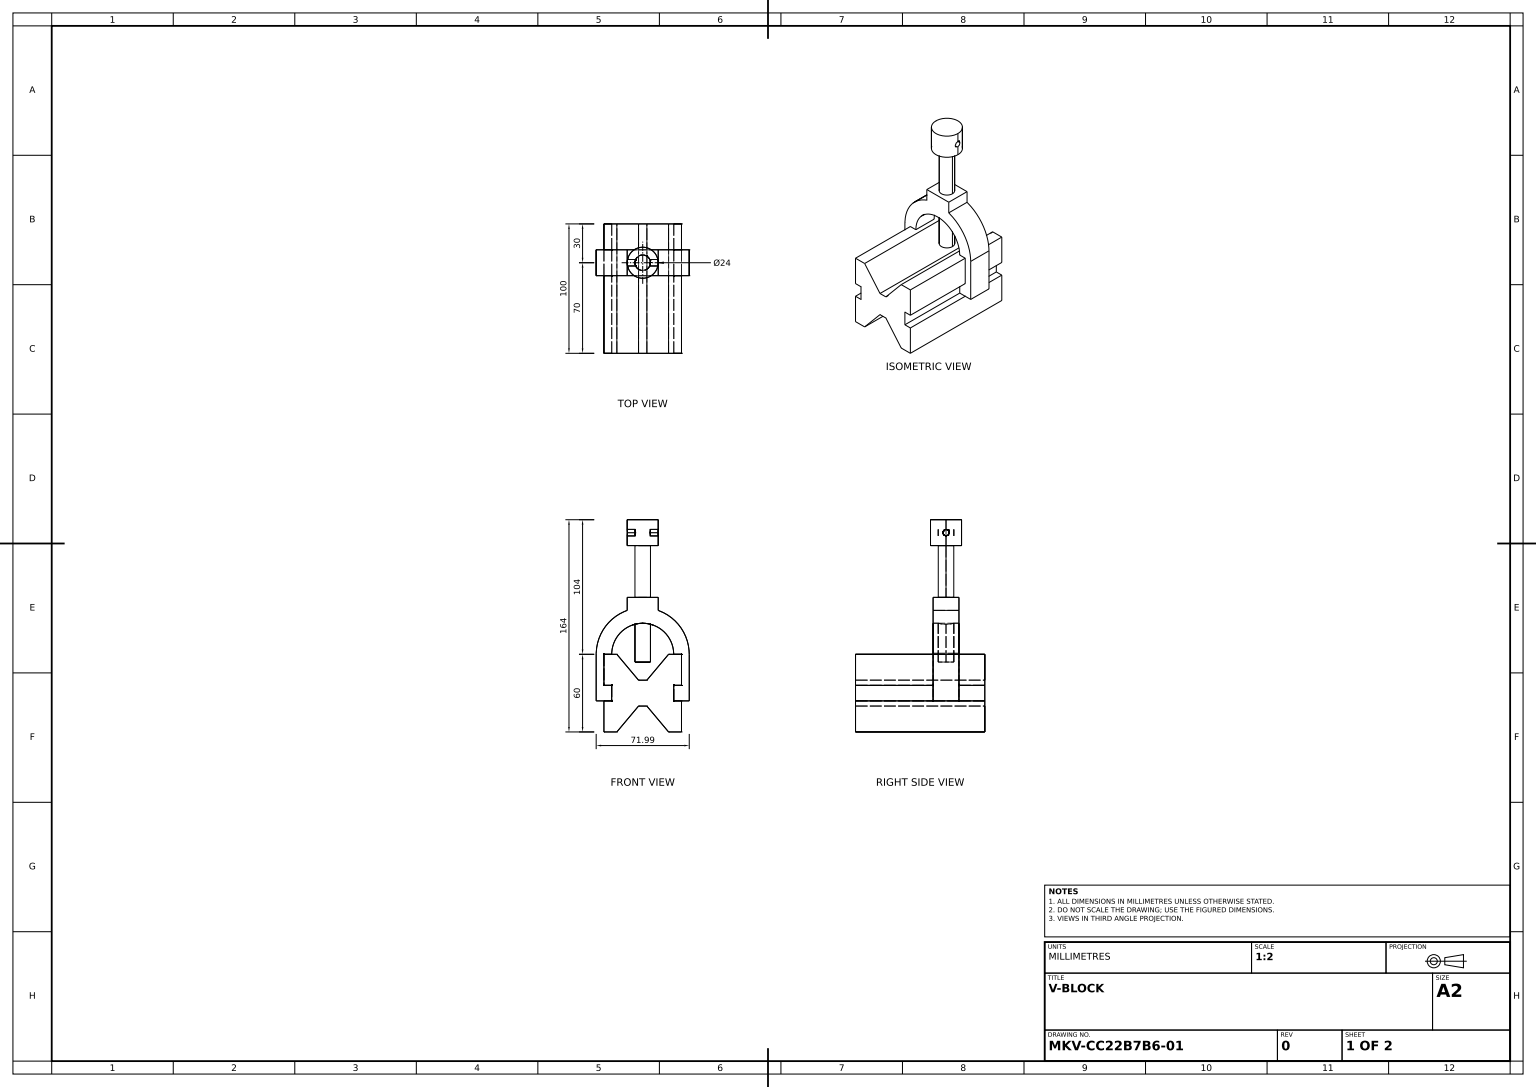
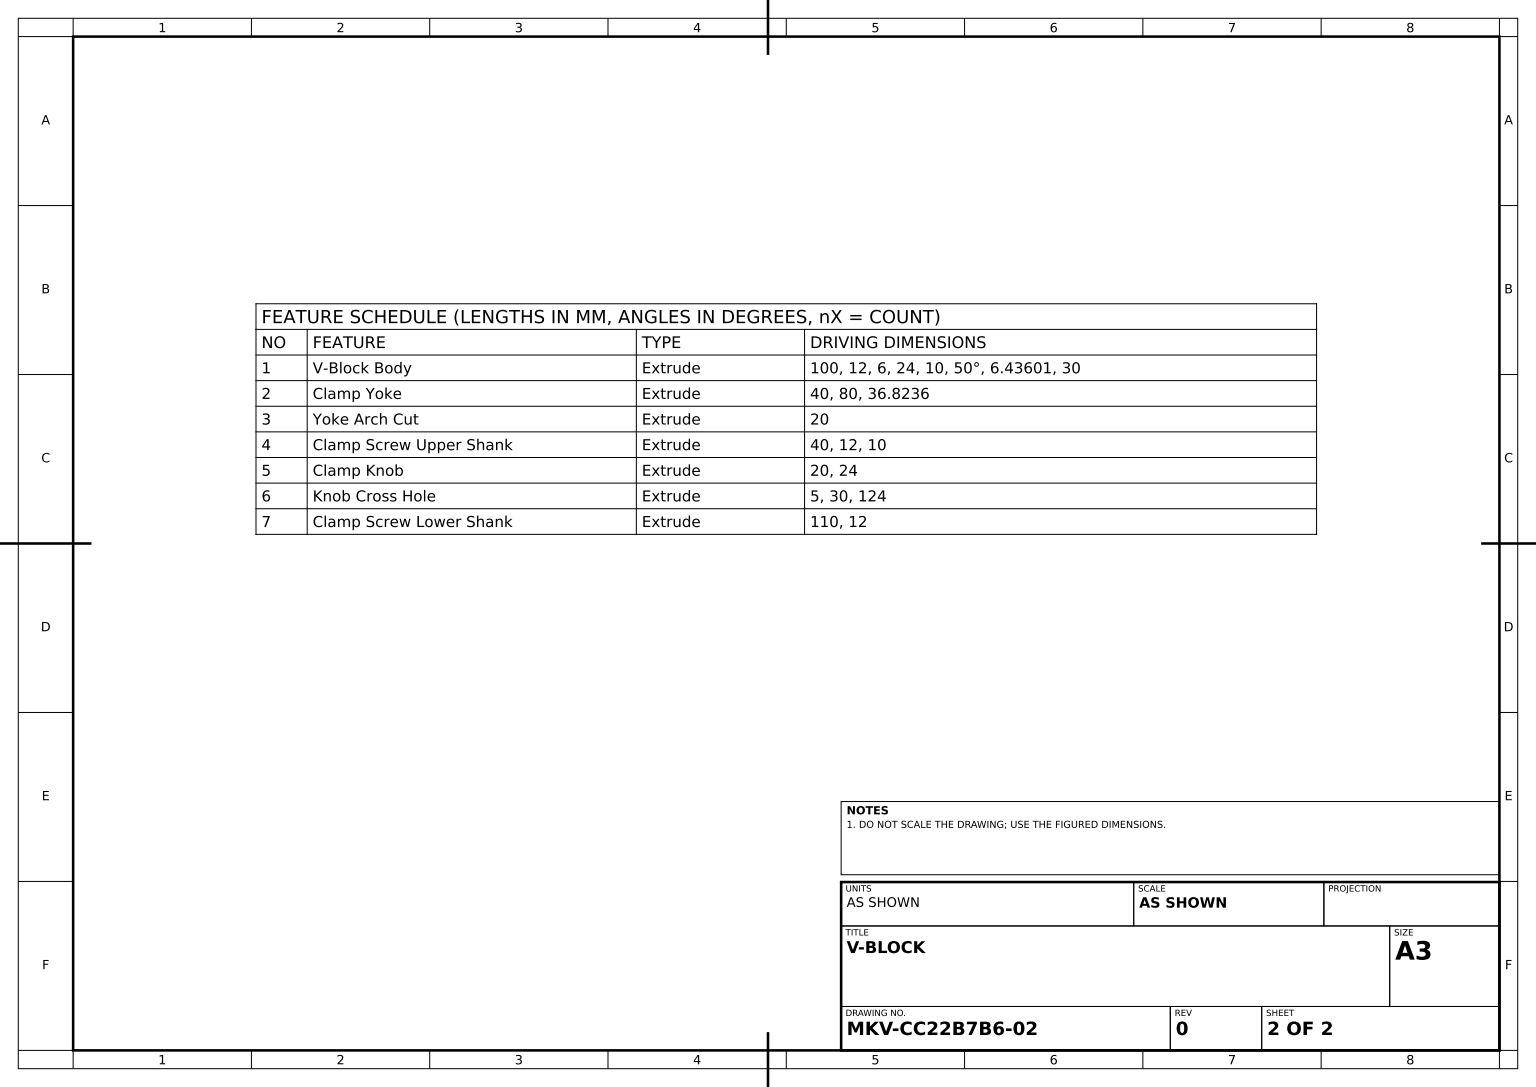
from build123d import *

# Parameters (mm, degrees)
V_BLOCK_BODY_DEPTH               = 100
CLAMP_YOKE_DEPTH                 = 40
YOKE_ARCH_CUT_DEPTH              = 20
CLAMP_SCREW_UPPER_SHANK_SKETCH_R = 6
CLAMP_SCREW_UPPER_SHANK_DEPTH    = 40
CLAMP_KNOB_SKETCH_R              = 12
CLAMP_KNOB_DEPTH                 = 20
KNOB_CROSS_HOLE_DEPTH            = 172.032160718
KNOB_CROSS_HOLE_DEPTH_BACK       = 172.032160718
KNOB_CROSS_HOLE_SKETCH_R         = 2.5
CLAMP_START                      = -110
CLAMP_SCREW_LOWER_SHANK_SKETCH_R = 6
CLAMP_SCREW_LOWER_SHANK_DEPTH    = 110


with BuildPart() as part:
    # V-Block Profile Sketch → V-Block Body (new body)
    with BuildSketch(Plane.XY):
        Polygon((-30, 30), (-20, 30), (-3.218007376, 10), (3.218007376, 10), (20, 30), (30, 30), (30, 6), (24, 6), (24, -6), (30, -6), (30, -30), (20, -30), (3.218007376, -10), (-3.218007376, -10), (-20, -30), (-30, -30), (-30, -6), (-24, -6), (-24, 6), (-30, 6), align=None)
    extrude(amount=V_BLOCK_BODY_DEPTH)

    # Clamp Yoke Sketch → Clamp Yoke (add)
    with BuildSketch(Plane(origin=(0, 0, 0), x_dir=(-1, 0, 0), z_dir=(0, 0, -1))):
        with BuildLine():
            Line((-24, -6), (-36, -6))
            Line((-36, -6), (-36, 30))
            ThreePointArc((-36, 30), (-29.393876913, 50.784609691), (-12, 63.941125497))
            Line((-12, 63.941125497), (-12, 74))
            Line((-12, 74), (12, 74))
            Line((12, 74), (12, 63.941125497))
            ThreePointArc((12, 63.941125497), (29.154199322, 51.11948536), (35.990578805, 30.823551635))
            Line((35.990578805, 30.823551635), (35.990578805, -6))
            Line((35.990578805, -6), (24, -6))
            Line((24, -6), (24, 6))
            Line((24, 6), (30, 6))
            Line((30, 6), (30, 30))
            Line((30, 30), (24, 30))
            ThreePointArc((24, 30), (0, 54), (-24, 30))
            Line((-24, 30), (-30, 30))
            Line((-30, 30), (-30, 6))
            Line((-30, 6), (-24, 6))
            Line((-24, 6), (-24, -6))
        make_face()
    extrude(amount=-CLAMP_YOKE_DEPTH)

    # Yoke Arch Cut Sketch → Yoke Arch Cut (cut)
    with BuildSketch(Plane(origin=(0, 0, 0), x_dir=(-1, 0, 0), z_dir=(0, 0, -1))):
        with BuildLine():
            Line((-30, -6), (-36, -6))
            Line((-36, -6), (-36, 30))
            ThreePointArc((-36, 30), (-29.393876913, 50.784609691), (-12, 63.941125497))
            Line((-12, 63.941125497), (-12, 74))
            Line((-12, 74), (12, 74))
            Line((12, 74), (12, 63.941125497))
            ThreePointArc((12, 63.941125497), (29.154199322, 51.11948536), (35.990578805, 30.823551635))
            Line((35.990578805, 30.823551635), (35.990578805, -6))
            Line((35.990578805, -6), (30, -6))
            Line((30, -6), (24, -6))
            Line((24, -6), (24, 6))
            Line((24, 6), (30, 6))
            Line((30, 6), (30, 30))
            Line((30, 30), (24, 30))
            ThreePointArc((24, 30), (0, 54), (-24, 30))
            Line((-24, 30), (-30, 30))
            Line((-30, 30), (-30, 6))
            Line((-30, 6), (-24, 6))
            Line((-24, 6), (-24, -6))
            Line((-24, -6), (-30, -6))
        make_face()
    extrude(amount=-YOKE_ARCH_CUT_DEPTH, mode=Mode.SUBTRACT)

    # Clamp Screw Upper Shank Sketch → Clamp Screw Upper Shank (add)
    with BuildSketch(Plane(origin=(0, 74, 0), x_dir=(1, 0, 0), z_dir=(0, 1, 0))):
        with Locations(Location((0, -30, 0), (0, 0, 180))):
            Circle(CLAMP_SCREW_UPPER_SHANK_SKETCH_R)
    extrude(amount=CLAMP_SCREW_UPPER_SHANK_DEPTH)

    # Clamp Knob Sketch → Clamp Knob (add)
    with BuildSketch(Plane(origin=(0, 114, 0), x_dir=(1, 0, 0), z_dir=(0, 1, 0))):
        with Locations(Location((0, -30, 0), (0, 0, 180))):
            Circle(CLAMP_KNOB_SKETCH_R)
    extrude(amount=CLAMP_KNOB_DEPTH)

    # Knob Cross Hole Sketch → Knob Cross Hole (cut, two sides: drawn at the far end of the back side and taken through both)
    with BuildSketch(Plane(origin=(0, 0, 0), x_dir=(0, 0, -1), z_dir=(1, 0, 0)).offset(-KNOB_CROSS_HOLE_DEPTH_BACK)):
        with Locations(Location((-30, 124, 0), (0, 0, 89.999999972))):
            Circle(KNOB_CROSS_HOLE_SKETCH_R)
    extrude(amount=KNOB_CROSS_HOLE_DEPTH + KNOB_CROSS_HOLE_DEPTH_BACK, mode=Mode.SUBTRACT)

    # Clamp Screw Lower Shank Sketch → Clamp Screw Lower Shank (add)
    with BuildSketch(Plane(origin=(0, 134, 0), x_dir=(1, 0, 0), z_dir=(0, 1, 0)).offset(CLAMP_START)):
        with Locations(Location((0, -30, 0), (0, 0, 180))):
            Circle(CLAMP_SCREW_LOWER_SHANK_SKETCH_R)
    extrude(amount=CLAMP_SCREW_LOWER_SHANK_DEPTH)


solid = part.part
